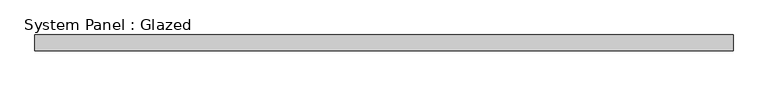
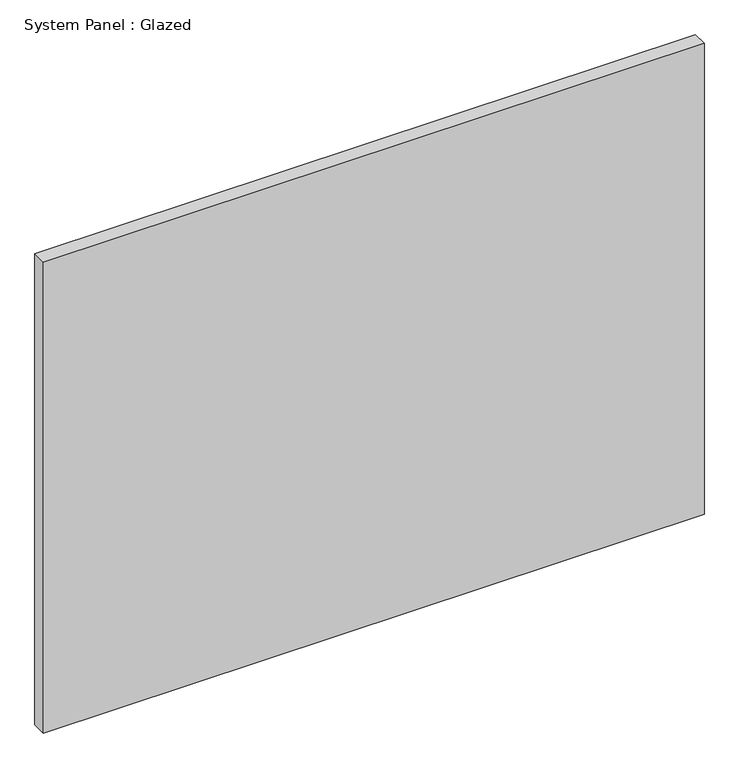
"""IFC4 building model written with IfcOpenShell, lengths in millimetres: plate geometry, System Panel : Glazed."""

from ifc_helpers import new_model, si_unit, origin, origin_with_axes, place, context, project, spatial, polyline, outline, extrude, source, transform, mapped, element, save


def system_panel_glazed_dd77c3d1(model_context):
    return source(origin(), model_context, "Body", "SweptSolid", [
        extrude(outline(polyline([(565.15, 19.05), (-565.15, 19.05), (-565.15, 44.45), (565.15, 44.45), (565.15, 19.05)])), origin_with_axes(), (0.0, 0.0, 1.0), 850.9),
    ])


if __name__ == "__main__":
    model = new_model("IFC4")
    model_context = context("Model", 3, world=origin())
    ifc_project = project(units=[si_unit("LENGTHUNIT", "METRE", prefix="MILLI")], contexts=[model_context])
    site = spatial("IfcSite", under=ifc_project)
    building = spatial("IfcBuilding", under=site)
    placement = place(None, origin())
    system_panel_glazed_shape = system_panel_glazed_dd77c3d1(model_context)
    element("IfcPlate", 1, ObjectType="System Panel : Glazed", at=placement, inside=building, context=model_context, shape_type="MappedRepresentation", body=[
        mapped(system_panel_glazed_shape, transform((0.0, 0.0, 0.0), x_axis=(1.0, 0.0, 0.0), y_axis=(0.0, 1.0, 0.0), z_axis=(0.0, 0.0, 1.0))),
    ])
    save(model, "model.ifc")

# Revit data of these elements
# Type "System Panel : Glazed"
#   Construction Type Id = "GSP4R"
#   Analytic Construction = "1/8 in Pilkington single glazing"
#   Visual Light Transmittance = 0.9
#   Solar Heat Gain Coefficient = 0.86
#   Heat Transfer Coefficient (U) = 1.18115 BTU/(h·ft²·°F)
# Element 1 (IfcPlate, "System Panel : Glazed")
#   Materials on its faces: "Glass"
# Materials
#   "Glass": class "Glass", colour RGB 0 128 192, transparency 0.75, Description = "Soda Lime Glass", Cost = 0
